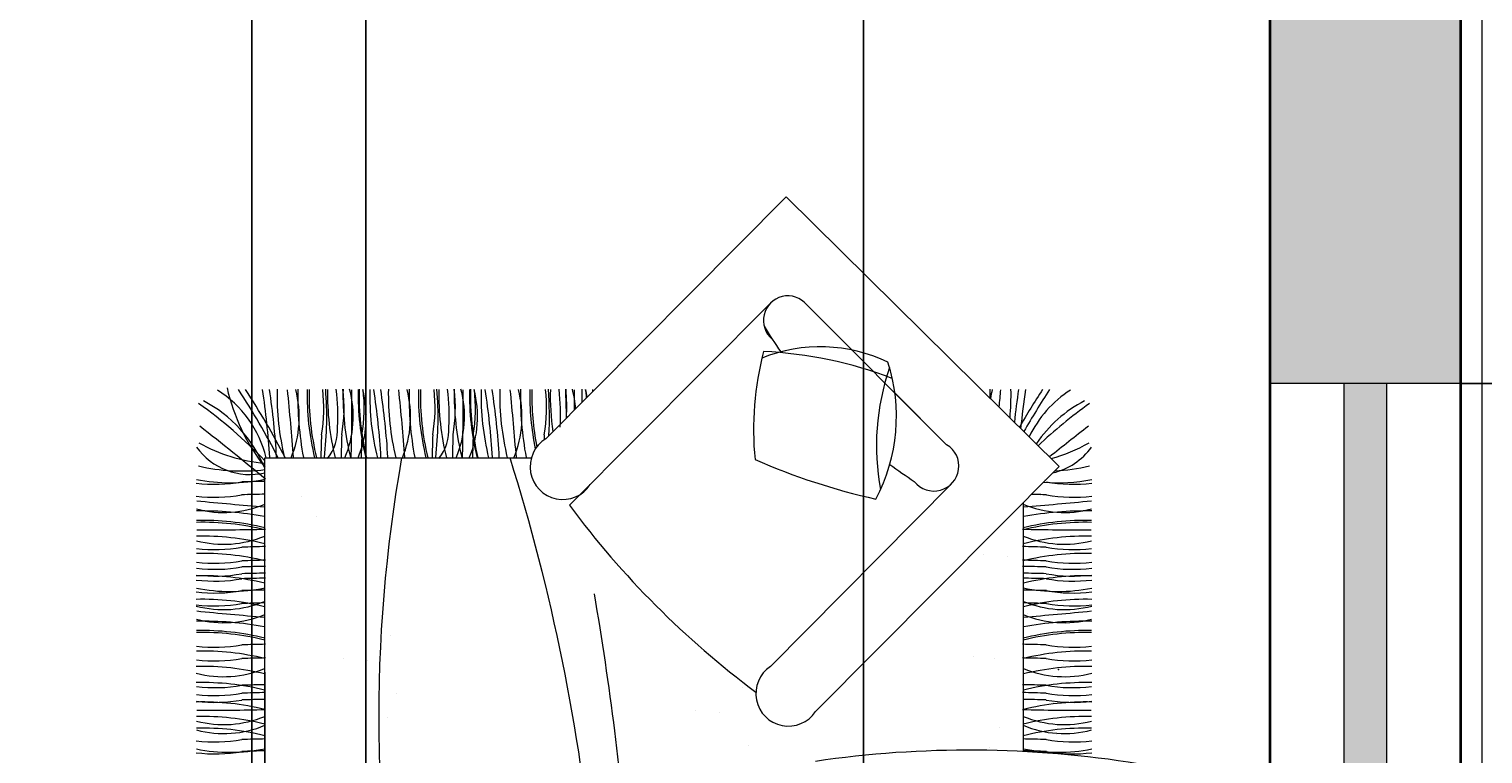
# Model space of a CAD drawing. Units: inches. Extents: x 311 to 815, y -527 to 136.
# Tile 12 of 21: x 655 to 723, y -403 to -368. Entities that reach past the tile are written whole.
import ezdxf

# ---------------------------------------------------------------- set-up
doc = ezdxf.new("R2010")
doc.units = ezdxf.units.IN
doc.header["$MEASUREMENT"] = 0
for name, color, linetype, lineweight in [('A-ANNO-DIMS', 1, 'Continuous', 18), ('A-FLOR-EDGE', 1, 'Continuous', 18), ('A-GLAZ-PATT', 5, 'Continuous', 13), ('A-WALL-PATT', 242, 'Continuous', 13), ('wall', 1, 'Continuous', 35), ('win', 5, 'Continuous', 18)]:
    doc.layers.add(name, color=color, linetype=linetype, lineweight=lineweight)
doc.layers.add('furniture', color=50, linetype='Continuous', lineweight=13, transparency=0.8)
doc.styles.get("Standard").update_dxf_attribs({"font": 'arial.ttf'})
doc.dimstyles.get("Standard").update_dxf_attribs({"dimtxt": 0.18, "dimasz": 0.18, "dimexe": 0.18, "dimexo": 0.0625, "dimgap": 0.09, "dimtad": 0, "dimtih": 1, "dimtoh": 1, "dimdec": 1, "dimzin": 0, "dimdsep": 46, "dimlunit": 4, "dimtxsty": 'Standard', "dimcen": 0.09, "dimadec": 0, "dimazin": 0, "dimtfac": 1, "dimtdec": 1, "dimtofl": 0, "dimtmove": 0, "dimatfit": 3, "dimfxl": 1, "dimtolj": 1, "dimtzin": 0, "dimarcsym": 0})

# ---------------------------------------------------------------- blocks, each defined once
blk = doc.blocks.new('WIN-60IN')
for p, q in [((9, 60), (0, 60)), ((3.5, 0), (3.5, 60)), ((5.5, 0), (5.5, 60)), ((9, 0), (0, 0))]:
    blk.add_line(p, q)
blk = doc.blocks.new('*D10')
at = {"layer": 'A-ANNO-DIMS', "color": 0, "lineweight": -2, "transparency": 16777216}
for p, q in [((722.385, -385.128), (731.503, -385.128)), ((731.323, -385.308), (731.323, -414.945)), ((731.323, -444.948), (731.323, -415.311)), ((722.385, -445.128), (731.503, -445.128))]:
    blk.add_line(p, q, dxfattribs=at)
at = {"layer": 'A-ANNO-DIMS', "color": 0, "transparency": 16777216}
for points in [[(731.293, -385.308), (731.353, -385.308), (731.323, -385.128)], [(731.293, -444.948), (731.353, -444.948), (731.323, -445.128)]]:
    blk.add_solid(points, dxfattribs=at)
at = {"layer": 'Defpoints', "color": 0, "transparency": 16777216}
for p in [(722.323, -385.128), (731.323, -385.128), (722.323, -445.128)]:
    blk.add_point(p, dxfattribs=at)
at = {"layer": 'A-ANNO-DIMS', "color": 0, "transparency": 16777216, "insert": (731.323, -415.128), "char_height": 0.18, "attachment_point": 5}
blk.add_mtext('\\A1;WINDOW 5\'-0" TYP.', dxfattribs=at)
blk = doc.blocks.new('*D28')
at = {"layer": 'A-ANNO-DIMS', "color": 0, "lineweight": -2, "transparency": 16777216}
for p, q in [((722.385, -322.628), (754.853, -322.628)), ((754.673, -322.808), (754.673, -353.695)), ((754.673, -384.948), (754.673, -354.061)), ((722.385, -385.128), (754.853, -385.128))]:
    blk.add_line(p, q, dxfattribs=at)
at = {"layer": 'A-ANNO-DIMS', "color": 0, "transparency": 16777216}
for points in [[(754.643, -322.808), (754.703, -322.808), (754.673, -322.628)], [(754.643, -384.948), (754.703, -384.948), (754.673, -385.128)]]:
    blk.add_solid(points, dxfattribs=at)
at = {"layer": 'Defpoints', "color": 0, "transparency": 16777216}
for p in [(722.323, -322.628), (722.323, -385.128), (754.673, -385.128)]:
    blk.add_point(p, dxfattribs=at)
at = {"layer": 'A-ANNO-DIMS', "color": 0, "transparency": 16777216, "insert": (754.673, -353.878), "char_height": 0.18, "attachment_point": 5}
blk.add_mtext('\\A1;5\'-2 1/2"', dxfattribs=at)
blk = doc.blocks.new('*D31')
at = {"layer": 'A-ANNO-DIMS', "color": 0, "lineweight": -2, "transparency": 16777216}
for p, q in [((670.696, -191.608), (670.696, -526.658)), ((694.164, -191.608), (694.164, -526.658)), ((670.876, -526.478), (681.83, -526.478)), ((693.984, -526.478), (683.03, -526.478))]:
    blk.add_line(p, q, dxfattribs=at)
at = {"layer": 'A-ANNO-DIMS', "color": 0, "transparency": 16777216}
for points in [[(670.876, -526.448), (670.876, -526.508), (670.696, -526.478)], [(693.984, -526.448), (693.984, -526.508), (694.164, -526.478)]]:
    blk.add_solid(points, dxfattribs=at)
at = {"layer": 'Defpoints', "color": 0, "transparency": 16777216}
for p in [(670.696, -191.545), (694.164, -191.545), (694.164, -526.478)]:
    blk.add_point(p, dxfattribs=at)
at = {"layer": 'A-ANNO-DIMS', "color": 0, "transparency": 16777216, "insert": (682.43, -526.478), "char_height": 0.18, "attachment_point": 5}
blk.add_mtext('\\A1;1\'-11 1/2"', dxfattribs=at)
blk = doc.blocks.new('*D37')
at = {"layer": 'A-ANNO-DIMS', "color": 0, "lineweight": -2, "transparency": 16777216}
for p, q in [((633.323, -348.19), (633.323, -526.658)), ((665.323, -348.19), (665.323, -526.658)), ((633.503, -526.478), (648.992, -526.478)), ((665.143, -526.478), (649.654, -526.478))]:
    blk.add_line(p, q, dxfattribs=at)
at = {"layer": 'A-ANNO-DIMS', "color": 0, "transparency": 16777216}
for points in [[(633.503, -526.448), (633.503, -526.508), (633.323, -526.478)], [(665.143, -526.448), (665.143, -526.508), (665.323, -526.478)]]:
    blk.add_solid(points, dxfattribs=at)
at = {"layer": 'Defpoints', "color": 0, "transparency": 16777216}
for p in [(633.323, -348.128), (665.323, -348.128), (665.323, -526.478)]:
    blk.add_point(p, dxfattribs=at)
at = {"layer": 'A-ANNO-DIMS', "color": 0, "transparency": 16777216, "insert": (649.323, -526.478), "char_height": 0.18, "attachment_point": 5}
blk.add_mtext('\\A1;2\'-8"', dxfattribs=at)

msp = doc.modelspace()

# ---------------------------------------------------------------- hatches: boundary and pattern name
at = {"layer": 'A-GLAZ-PATT'}
h = msp.add_hatch(color=256, dxfattribs=at)
h.dxf.hatch_style = 1
h.paths.add_polyline_path([(415.823, -202.128), (413.823, -202.128), (413.823, -262.128), (415.823, -262.128)])
h.paths.add_polyline_path([(415.823, -390.84), (413.823, -390.84), (413.823, -450.84), (415.823, -450.84)])
h.paths.add_polyline_path([(415.823, -311.568), (413.823, -311.568), (413.823, -335.568), (415.823, -335.568)])
h.paths.add_polyline_path([(509.323, -476.628), (449.323, -476.628), (449.323, -478.628), (509.323, -478.628)])
h.paths.add_polyline_path([(606.823, -476.628), (582.823, -476.628), (582.823, -478.628), (606.823, -478.628)])
h.paths.add_polyline_path([(678.823, -476.628), (654.823, -476.628), (654.823, -478.628), (678.823, -478.628)])
h.paths.add_polyline_path([(718.823, -385.128), (716.823, -385.128), (716.823, -445.128), (718.823, -445.128)])
h.paths.add_polyline_path([(718.823, -262.628), (716.823, -262.628), (716.823, -322.628), (718.823, -322.628)])
h.paths.add_polyline_path([(718.823, -140.128), (716.823, -140.128), (716.823, -200.128), (718.823, -200.128)])
h.paths.add_polyline_path([(718.823, -18.128), (716.823, -18.128), (716.823, -42.128), (718.823, -42.128)])
h.paths.add_polyline_path([(686.823, 18.372), (626.823, 18.372), (626.823, 16.372), (686.823, 16.372)])
h.paths.add_polyline_path([(581.823, 18.372), (557.823, 18.372), (557.823, 16.372), (581.823, 16.372)])
h.paths.add_polyline_path([(509.323, 18.372), (449.323, 18.372), (449.323, 16.372), (509.323, 16.372)])
at = {"layer": 'A-WALL-PATT'}
h = msp.add_hatch(color=256, dxfattribs=at)
h.dxf.hatch_style = 1
h.paths.add_polyline_path([(557.823, 21.872), (509.323, 21.872), (509.323, 12.872), (539.323, 12.872), (539.323, -112.128), (548.323, -112.128), (548.323, -58.628), (557.823, -58.628), (557.823, -49.628), (548.323, -49.628), (548.323, 12.872), (557.823, 12.872)])
h.paths.add_polyline_path([(449.323, 21.872), (410.323, 21.872), (410.323, -15.128), (419.323, -15.128), (419.323, 12.872), (449.323, 12.872)])
h.paths.add_polyline_path([(626.823, 21.872), (581.823, 21.872), (581.823, 12.872), (591.323, 12.872), (591.323, -49.628), (581.823, -49.628), (581.823, -58.628), (591.323, -58.628), (591.323, -112.128), (600.323, -112.128), (600.323, 12.872), (626.823, 12.872)])
h.paths.add_polyline_path([(722.323, 21.872), (686.823, 21.872), (686.823, 12.872), (713.323, 12.872), (713.323, -18.128), (722.323, -18.128)])
h.paths.add_polyline_path([(722.323, -42.128), (713.323, -42.128), (713.323, -73.128), (722.323, -73.128)])
h.paths.add_polyline_path([(501.323, -103.128), (419.323, -103.128), (419.323, -75.128), (410.323, -75.128), (410.323, -126.628), (419.323, -126.628), (419.323, -112.128), (492.323, -112.128), (492.323, -143.128), (501.323, -143.128)])
h.paths.add_polyline_path([(548.323, -165.128), (419.323, -165.128), (419.323, -150.628), (410.323, -150.628), (410.323, -202.128), (419.323, -202.128), (419.323, -174.128), (548.323, -174.128)])
h.paths.add_polyline_path([(722.323, -103.128), (636.323, -103.128), (636.323, -112.128), (713.323, -112.128), (713.323, -140.128), (722.323, -140.128)])
h.paths.add_polyline_path([(548.323, -210.128), (539.323, -210.128), (539.323, -290.128), (419.323, -290.128), (419.323, -262.128), (410.323, -262.128), (410.323, -311.568), (419.323, -311.568), (419.323, -299.128), (469.323, -299.128), (469.323, -348.128), (443.323, -348.128), (443.323, -357.128), (478.323, -357.128), (478.323, -299.128), (548.323, -299.128)])
h.paths.add_polyline_path([(722.323, -200.128), (713.323, -200.128), (713.323, -228.128), (609.323, -228.128), (609.323, -237.128), (713.323, -237.128), (713.323, -262.628), (722.323, -262.628)])
h.paths.add_polyline_path([(722.323, -322.628), (713.323, -322.628), (713.323, -348.128), (633.323, -348.128), (633.323, -357.128), (713.323, -357.128), (713.323, -385.128), (722.323, -385.128)])
h.paths.add_polyline_path([(419.323, -335.568), (410.323, -335.568), (410.323, -390.84), (419.323, -390.84)])
h.paths.add_polyline_path([(419.323, -450.84), (410.323, -450.84), (410.323, -482.128), (449.323, -482.128), (449.323, -473.128), (419.323, -473.128)])
h.paths.add_polyline_path([(582.823, -473.128), (548.323, -473.128), (548.323, -348.128), (539.323, -348.128), (539.323, -473.128), (509.323, -473.128), (509.323, -482.128), (582.823, -482.128)])
h.paths.add_polyline_path([(722.323, -445.128), (713.323, -445.128), (713.323, -473.128), (678.823, -473.128), (678.823, -482.128), (722.323, -482.128)])

# ---------------------------------------------------------------- linework, layer by layer
at = {"layer": 'A-FLOR-EDGE'}
msp.add_line((723.323, -483.128), (723.323, 22.872), dxfattribs=at)
at = {"layer": 'furniture'}
for p, q in [((690.515, -376.331), (679.179, -387.73)), ((703.381, -389.035), (690.515, -376.331)), ((680.299, -390.867), (689.78, -381.34)), ((698.077, -388.013), (691.477, -381.413)), ((693.622, -383.558), (691.477, -381.413)), ((698.077, -388.013), (695.637, -385.572)), ((670.738, -386.61), (670.738, -386.61)), ((670.763, -386.914), (670.763, -386.914)), ((675.984, -386.61), (675.984, -386.61)), ((676.009, -386.914), (676.009, -386.914)), ((665.936, -452.501), (665.936, -388.632)), ((665.936, -388.632), (678.498, -388.632)), ((703.381, -389.035), (691.898, -400.584)), ((664.928, -389.647), (664.928, -389.647)), ((664.928, -389.647), (664.928, -389.647)), ((664.928, -389.647), (664.928, -389.647)), ((698.312, -389.851), (689.768, -398.454)), ((702.695, -389.647), (702.695, -389.647)), ((702.695, -389.647), (702.695, -389.647)), ((702.695, -389.647), (702.695, -389.647)), ((665.118, -390.42), (665.118, -390.42)), ((665.118, -390.42), (665.118, -390.42)), ((665.118, -390.42), (665.118, -390.42)), ((667.679, -390.438), (667.679, -390.438)), ((702.505, -390.42), (702.505, -390.42)), ((702.505, -390.42), (702.505, -390.42)), ((702.505, -390.42), (702.505, -390.42)), ((701.687, -390.738), (701.687, -402.463)), ((668.364, -391.4), (668.364, -391.4)), ((702.02, -392.108), (702.02, -392.108)), ((702.02, -392.108), (702.02, -392.108)), ((699.795, -393.186), (699.795, -393.186)), ((700.926, -393.268), (700.926, -393.268)), ((702.292, -394.841), (702.292, -394.841)), ((701.893, -395.978), (701.893, -395.978)), ((671.848, -397.008), (671.848, -397.008)), ((671.848, -397.008), (671.848, -397.008)), ((669.623, -398.087), (669.623, -398.087)), ((670.754, -398.168), (670.754, -398.168)), ((699.345, -397.989), (699.345, -397.989)), ((700.315, -398.064), (700.315, -398.064)), ((665.936, -398.727), (665.936, -452.501)), ((701.706, -398.558), (701.706, -398.558)), ((703.581, -398.374), (703.581, -398.374)), ((688.443, -399.459), (688.443, -399.459)), ((688.443, -399.459), (688.443, -399.459)), ((672.12, -399.742), (672.12, -399.742)), ((703.118, -400.15), (703.118, -400.15)), ((671.721, -400.878), (671.721, -400.878)), ((686.218, -400.537), (686.218, -400.537)), ((687.349, -400.619), (687.349, -400.619)), ((700.569, -401.314), (700.569, -401.314)), ((688.714, -402.192), (688.714, -402.192)), ((700.107, -402.267), (700.107, -402.267)), ((703.247, -401.667), (703.247, -401.667))]:
    msp.add_line(p, q, dxfattribs=at)
for centre, radius, start, end in [((690.595, -382.156), 1.153, 40.10925, 229.89075), ((708.815, -370.777), 22.581, 211.08667, 214.72696), ((703.487, -387.301), 14.512, 165.30685, 185.5663), ((692.116, -390.803), 7.4, 64.45006, 111.76991), ((688.518, -403.195), 19.597, 69.08153, 87.27682), ((687.418, -386.682), 8.293, 332.0126, 17.9429), ((705.992, -388.053), 11.224, 160.90051, 190.65125), ((660.88, -389.906), 5.282, 13.99349, 57.72877), ((673.427, -383.198), 9.516, 192.95229, 218.0769), ((634.552, -405.131), 36.02, 27.26685, 33.17806), ((634.877, -405.123), 36.02, 27.26685, 33.17806), ((631.241, -390.664), 34.984, 3.36442, 8.62286), ((631.566, -390.656), 34.984, 3.36442, 8.62286), ((678.75, -385.694), 12.239, 178.63307, 193.85735), ((524.875, -399.862), 142.863, 4.51462, 5.80171), ((662.542, -386.698), 5.018, 337.30984, 14.86132), ((683.738, -385.682), 16.251, 179.01954, 190.40392), ((680.168, -385.7), 12.239, 178.63307, 193.85735), ((680.259, -385.7), 12.239, 178.63307, 193.85735), ((661.452, -386.276), 7.265, 349.93491, 6.88295), ((652.323, -386.702), 16.533, 353.37018, 4.50636), ((681.133, -385.697), 12.239, 178.63307, 193.85735), ((658.054, -386.674), 11.324, 357.44348, 6.44133), ((662.407, -386.273), 7.265, 349.93491, 6.88295), ((681.857, -385.691), 12.239, 178.63307, 193.85735), ((665.085, -386.688), 5.018, 337.30984, 14.86132), ((565.264, -386.153), 104.775, 358.62796, 0.39341), ((665.7, -386.696), 5.018, 337.30984, 14.86132), ((682.576, -385.699), 12.239, 178.63307, 193.85735), ((682.617, -385.693), 12.239, 178.63307, 193.85735), ((663.355, -386.28), 7.265, 349.93491, 6.88295), ((683.123, -385.704), 12.239, 178.63307, 193.85735), ((636.487, -390.664), 34.984, 3.36442, 8.62286), ((636.813, -390.656), 34.984, 3.36442, 8.62286), ((683.997, -385.694), 12.239, 178.63307, 193.85735), ((530.121, -399.862), 142.863, 4.51462, 5.80171), ((667.789, -386.698), 5.018, 337.30984, 14.86132), ((688.984, -385.682), 16.251, 179.01954, 190.40392), ((685.415, -385.7), 12.239, 178.63307, 193.85735), ((685.506, -385.7), 12.239, 178.63307, 193.85735), ((666.699, -386.276), 7.265, 349.93491, 6.88295), ((657.57, -386.702), 16.533, 353.37018, 4.50636), ((686.379, -385.697), 12.239, 178.63307, 193.85735), ((663.301, -386.674), 11.324, 357.44348, 6.44133), ((667.654, -386.273), 7.265, 349.93491, 6.88295), ((687.104, -385.691), 12.239, 178.63307, 193.85735), ((670.332, -386.688), 5.018, 337.30984, 14.86132), ((570.51, -386.153), 104.775, 358.62796, 0.39341), ((670.947, -386.696), 5.018, 337.30984, 14.86132), ((687.823, -385.699), 12.239, 178.63307, 193.85735), ((687.864, -385.693), 12.239, 178.63307, 193.85735), ((668.602, -386.28), 7.265, 349.93491, 6.88295), ((688.37, -385.704), 12.239, 178.63307, 193.85735), ((641.74, -390.664), 34.984, 3.36442, 8.62286), ((642.065, -390.656), 34.984, 3.36442, 8.62286), ((689.249, -385.694), 12.239, 178.63307, 193.85735), ((535.374, -399.862), 142.863, 4.51462, 5.80171), ((673.041, -386.698), 5.018, 337.30984, 14.86132), ((694.236, -385.682), 16.251, 179.01954, 190.40392), ((690.667, -385.7), 12.239, 178.63307, 191.83019), ((690.758, -385.7), 12.239, 178.63307, 191.35191), ((671.951, -386.276), 7.265, 349.93491, 6.88295), ((662.822, -386.702), 16.533, 356.96769, 4.50636), ((691.632, -385.697), 12.239, 178.63307, 187.97978), ((668.553, -386.674), 11.324, 357.44348, 6.44133), ((692.356, -385.691), 12.239, 178.63307, 184.92383), ((672.906, -386.273), 7.265, 356.24526, 6.88295), ((675.584, -386.688), 5.018, 4.27566, 14.86132), ((575.763, -386.153), 104.775, 359.8849, 0.39341), ((693.116, -385.693), 12.239, 178.63307, 181.52384), ((676.199, -386.696), 5.018, 10.65917, 14.86132), ((673.854, -386.28), 7.265, 3.81728, 6.88295), ((693.622, -385.704), 12.239, 178.63307, 179.10459), ((683.886, -385.682), 16.251, 359.47531, 0.98046), ((705.081, -386.698), 5.018, 165.13868, 170.07522), ((842.749, -399.862), 142.863, 174.19829, 174.52363), ((688.873, -385.694), 12.239, 355.05376, 1.36693), ((736.057, -390.656), 34.984, 171.37714, 173.92031), ((732.746, -405.123), 36.02, 146.82194, 150.13556), ((736.383, -390.664), 34.984, 171.37714, 174.38877), ((733.071, -405.131), 36.02, 146.82194, 150.50261), ((706.743, -389.906), 5.282, 122.27123, 154.62744), ((650.334, -403.686), 21.587, 43.716, 54.68473), ((660.203, -391.447), 6.189, 22.11811, 62.69671), ((707.421, -391.447), 6.189, 117.30329, 145.70162), ((717.29, -403.686), 21.587, 125.31527, 133.64566), ((602.458, -465.747), 99.132, 50.15682, 52.45592), ((667.182, -387.301), 2.188, 321.65644, 3.17437), ((672.428, -387.301), 2.188, 321.65644, 3.17437), ((765.166, -465.747), 99.132, 127.54408, 128.89007), ((749.601, -390.107), 81.037, 178.18909, 178.97752), ((750.556, -390.104), 81.037, 178.18909, 178.97752), ((751.504, -390.11), 81.037, 178.18909, 178.97752), ((754.848, -390.107), 81.037, 178.18909, 178.97752), ((755.803, -390.104), 81.037, 178.18909, 178.97752), ((756.751, -390.11), 81.037, 178.18909, 178.97752), ((679.986, -389.047), 1.544, 121.46934, 326.90762), ((760.1, -390.107), 81.037, 178.18909, 178.3576), ((665.244, -386.29), 3.126, 215.90571, 282.80539), ((666.483, -381.562), 7.336, 240.13503, 265.72435), ((697.482, -389.023), 1.172, 217.67477, 59.51812), ((701.14, -381.562), 7.336, 284.67923, 299.86497), ((702.38, -386.29), 3.126, 282.97771, 324.09429), ((664.838, -380.423), 8.827, 256.72146, 277.14908), ((741.561, -400.92), 70.258, 169.92753, 191.22459), ((587.613, -416.937), 94.235, 5.44209, 17.47988), ((701.505, -360.27), 31.049, 246.33709, 257.41765), ((708.815, -370.777), 22.581, 233.54543, 237.11437), ((702.786, -380.423), 8.827, 272.5322, 283.27854), ((663.575, -382.613), 7.265, 263.11705, 280.06509), ((664.295, -381.666), 8.138, 258.75453, 281.58879), ((667.406, -470.762), 81.037, 91.02248, 91.81091), ((703.329, -381.666), 8.138, 265.1756, 281.24547), ((704.048, -382.613), 7.265, 259.93491, 276.88295), ((663.574, -383.22), 7.265, 263.11705, 280.06509), ((677.166, -248.52), 142.863, 264.19829, 265.48538), ((667.404, -471.369), 81.037, 91.02248, 91.81091), ((690.457, -248.52), 142.863, 274.51462, 275.80171), ((700.219, -471.369), 81.037, 88.18909, 88.67093), ((704.05, -383.22), 7.265, 259.93491, 276.88295), ((662.987, -407.383), 16.251, 79.59608, 90.98046), ((664.003, -386.187), 5.018, 255.13868, 292.69016), ((714.586, -365.399), 42.711, 216.60494, 233.33873), ((703.621, -386.187), 5.018, 247.30984, 284.86132), ((704.637, -407.383), 16.251, 89.01954, 100.40392), ((663.005, -403.813), 12.239, 76.14265, 91.36693), ((663.005, -403.904), 12.239, 76.14265, 91.36693), ((663.458, -287.246), 104.775, 269.60659, 271.37204), ((704.166, -287.246), 104.775, 268.62796, 270.39341), ((704.619, -403.813), 12.239, 88.63307, 103.85735), ((704.619, -403.904), 12.239, 88.63307, 103.85735), ((663.004, -404.559), 12.239, 76.14265, 91.36693), ((664, -387.683), 5.018, 255.13868, 292.69016), ((703.623, -387.683), 5.018, 247.30984, 284.86132), ((704.62, -404.559), 12.239, 88.63307, 103.85735), ((663.581, -385.687), 7.265, 263.11705, 280.06509), ((663.002, -405.368), 12.239, 76.14265, 91.36693), ((667.411, -473.836), 81.037, 91.02248, 91.81091), ((700.212, -473.836), 81.037, 88.18909, 88.97752), ((704.622, -405.368), 12.239, 88.63307, 103.85735), ((704.043, -385.687), 7.265, 259.93491, 276.88295), ((663.578, -386.617), 7.265, 263.11705, 280.06509), ((663.579, -386.329), 7.265, 263.11705, 280.06509), ((667.408, -475.087), 81.037, 91.02248, 91.81091), ((667.409, -474.766), 81.037, 91.02248, 91.81091), ((667.41, -474.479), 81.037, 91.02248, 91.81091), ((700.214, -474.479), 81.037, 88.18909, 88.97752), ((700.215, -474.766), 81.037, 88.18909, 88.97752), ((700.216, -475.087), 81.037, 88.18909, 88.97752), ((704.044, -386.329), 7.265, 259.93491, 276.88295), ((704.045, -386.617), 7.265, 259.93491, 276.88295), ((663.577, -387.173), 7.265, 263.11705, 280.06509), ((663.578, -386.938), 7.265, 263.11705, 280.06509), ((662.999, -406.421), 12.239, 76.14265, 91.36693), ((664.295, -386.786), 8.138, 258.75453, 281.58879), ((667.407, -475.322), 81.037, 91.02248, 91.81091), ((700.216, -475.322), 81.037, 88.18909, 88.97752), ((704.625, -406.421), 12.239, 88.63307, 103.85735), ((703.329, -386.786), 8.138, 258.41121, 281.24547), ((704.046, -386.938), 7.265, 259.93491, 276.88295), ((704.047, -387.173), 7.265, 259.93491, 276.88295), ((662.996, -407.531), 12.239, 76.14265, 91.36693), ((663.575, -387.733), 7.265, 263.11705, 280.06509), ((663.992, -390.76), 5.018, 255.13868, 292.69016), ((667.406, -475.882), 81.037, 91.02248, 91.81091), ((537.566, -419.76), 146.015, 4.61959, 9.75131), ((700.218, -475.882), 81.037, 88.18909, 88.97752), ((704.628, -407.531), 12.239, 88.63307, 103.85735), ((703.631, -390.76), 5.018, 247.30984, 284.86132), ((704.048, -387.733), 7.265, 259.93491, 276.88295), ((663.574, -388.34), 7.265, 263.11705, 280.06509), ((664.003, -391.378), 5.018, 255.13868, 292.69016), ((677.166, -253.711), 142.863, 264.19829, 265.48538), ((667.404, -476.489), 81.037, 91.02248, 91.81091), ((700.219, -476.489), 81.037, 88.18909, 88.97752), ((703.621, -391.378), 5.018, 247.30984, 284.86132), ((690.457, -253.711), 142.863, 274.51462, 275.80171), ((704.05, -388.34), 7.265, 259.93491, 276.88295), ((662.987, -412.574), 16.251, 79.59608, 90.98046), ((663.005, -409.005), 12.239, 76.14265, 91.36693), ((704.619, -409.005), 12.239, 88.63307, 103.85735), ((704.637, -412.574), 16.251, 89.01954, 100.40392), ((663.581, -390.289), 7.265, 263.11705, 280.06509), ((663.005, -409.096), 12.239, 76.14265, 91.36693), ((667.411, -478.438), 81.037, 91.02248, 91.81091), ((700.212, -478.438), 81.037, 88.18909, 88.97752), ((704.619, -409.096), 12.239, 88.63307, 103.85735), ((704.043, -390.289), 7.265, 259.93491, 276.88295), ((663.579, -390.931), 7.265, 263.11705, 280.06509), ((663.002, -409.969), 12.239, 76.14265, 91.36693), ((667.41, -479.08), 81.037, 91.02248, 91.81091), ((700.214, -479.08), 81.037, 88.18909, 88.97752), ((704.622, -409.969), 12.239, 88.63307, 103.85735), ((704.044, -390.931), 7.265, 259.93491, 276.88295), ((662.996, -410.693), 12.239, 76.14265, 91.36693), ((663.992, -393.921), 5.018, 255.13868, 292.69016), ((690.619, -399.733), 1.536, 123.6335, 326.3665), ((704.628, -410.693), 12.239, 88.63307, 103.85735), ((703.631, -393.921), 5.018, 247.30984, 284.86132), ((662.997, -411.454), 12.239, 76.14265, 91.36693), ((663.584, -392.191), 7.265, 263.11705, 280.06509), ((667.415, -480.341), 81.037, 91.02248, 91.81091), ((700.209, -480.341), 81.037, 88.18909, 88.97752), ((704.626, -411.454), 12.239, 88.63307, 103.85735), ((704.039, -392.191), 7.265, 259.93491, 276.88295), ((663.578, -392.884), 7.265, 263.11705, 280.06509), ((662.999, -412.367), 12.239, 76.14265, 91.36693), ((663.578, -392.563), 7.265, 263.11705, 280.06509), ((667.408, -481.033), 81.037, 91.02248, 91.81091), ((667.409, -480.712), 81.037, 91.02248, 91.81091), ((700.215, -480.712), 81.037, 88.18909, 88.97752), ((700.216, -481.033), 81.037, 88.18909, 88.97752), ((704.625, -412.367), 12.239, 88.63307, 103.85735), ((704.045, -392.563), 7.265, 259.93491, 276.88295), ((704.046, -392.884), 7.265, 259.93491, 276.88295), ((663.004, -413.053), 12.239, 76.14265, 91.36693), ((664, -396.177), 5.018, 255.13868, 292.69016), ((663.458, -295.741), 104.775, 269.60659, 271.37204), ((704.166, -295.741), 104.775, 268.62796, 270.39341), ((703.623, -396.177), 5.018, 247.30984, 284.86132), ((704.62, -413.053), 12.239, 88.63307, 103.85735), ((663.008, -413.6), 12.239, 76.14265, 91.36693), ((664.005, -396.599), 5.018, 255.13868, 292.69016), ((703.618, -396.599), 5.018, 247.30984, 284.86132), ((704.615, -413.6), 12.239, 88.63307, 103.85735), ((663.577, -394.748), 7.265, 263.11705, 280.06509), ((667.407, -482.897), 81.037, 91.02248, 91.81091), ((700.216, -482.897), 81.037, 88.18909, 88.97752), ((704.047, -394.748), 7.265, 259.93491, 276.88295), ((663.575, -395.308), 7.265, 263.11705, 280.06509), ((664.295, -394.361), 8.138, 258.75453, 281.58879), ((667.406, -483.457), 81.037, 91.02248, 91.81091), ((699.135, -452.295), 49.897, 80.80787, 98.3514), ((700.218, -483.457), 81.037, 88.18909, 88.97752), ((703.329, -394.361), 8.138, 258.41121, 281.24547), ((704.048, -395.308), 7.265, 259.93491, 276.88295)]:
    msp.add_arc(centre, radius, start, end, dxfattribs=at)
msp.add_point((703.358, -398.596), dxfattribs=at)
at = {"layer": 'wall'}
for p, q in [((722.323, -482.128), (722.323, -103.128)), ((713.323, -473.128), (713.323, -357.128))]:
    msp.add_line(p, q, dxfattribs=at)

# ---------------------------------------------------------------- block references
at = {"layer": 'win'}
msp.add_blockref('WIN-60IN', (713.323, -445.128), dxfattribs=at)

# ---------------------------------------------------------------- dimensions: what is measured, and where the dimension line sits
at = {"layer": 'A-ANNO-DIMS'}
for base, p1, p2, picture, middle in [((694.164, -526.478), (670.696, -191.545), (694.164, -191.545), '*D31', (682.43, -526.478)), ((665.323, -526.478), (633.323, -348.128), (665.323, -348.128), '*D37', (649.323, -526.478))]:
    dim = msp.add_linear_dim(base=base, p1=p1, p2=p2, dimstyle='Standard', override={"dimdec": 1, "dimlfac": 1, "dimrnd": 0, "dimzin": 1, "dimdsep": 46, "dimlunit": 4, "dimfrac": 2}, dxfattribs=at)
    dim.commit()
    dim.dimension.update_dxf_attribs({"geometry": picture, "text_midpoint": middle})
dim = msp.add_linear_dim(base=(754.673, -385.128), p1=(722.323, -322.628), p2=(722.323, -385.128), angle=90, dimstyle='Standard', override={"dimdec": 1, "dimlfac": 1, "dimrnd": 0, "dimzin": 1, "dimdsep": 46, "dimlunit": 4, "dimfrac": 2}, dxfattribs=at)
dim.commit()
dim.dimension.update_dxf_attribs({"geometry": '*D28', "text_midpoint": (754.673, -353.878)})
dim = msp.add_linear_dim(base=(731.323, -385.128), p1=(722.323, -445.128), p2=(722.323, -385.128), angle=90, text='WINDOW <> TYP.', dimstyle='Standard', override={"dimdec": 1, "dimlfac": 1, "dimrnd": 0, "dimzin": 1, "dimdsep": 46, "dimlunit": 4, "dimfrac": 2}, dxfattribs=at)
dim.commit()
dim.dimension.update_dxf_attribs({"geometry": '*D10', "text_midpoint": (731.323, -415.128)})

doc.saveas('drawing.dxf')
